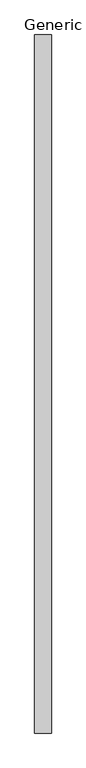
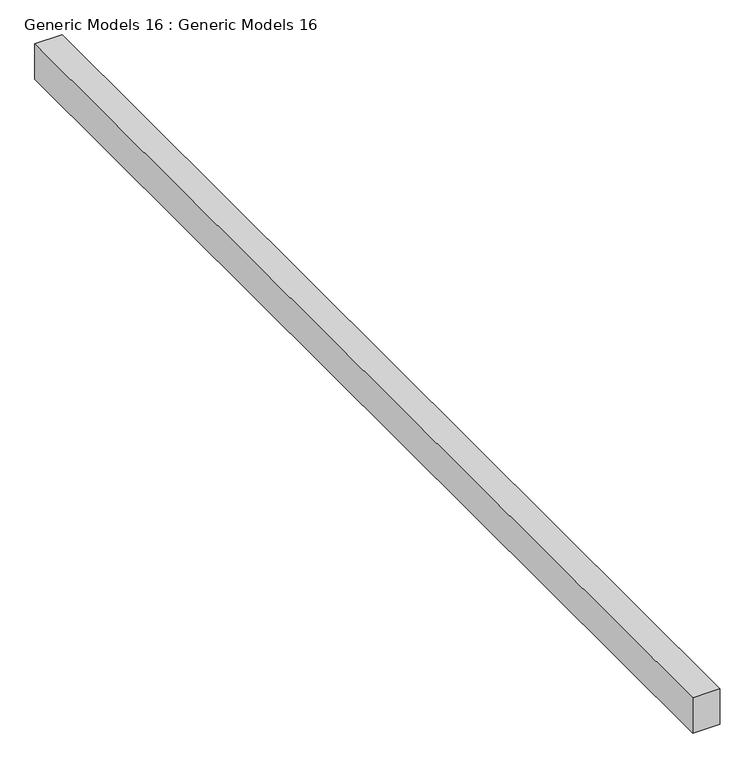
"""IFC4 building model written with IfcOpenShell, lengths in millimetres: proxy geometry, Generic Models 16 : Generic Models 16."""

from ifc_helpers import new_model, si_unit, frame, origin, place, context, project, spatial, polyline, outline, extrude, source, transform, mapped, element, save


def generic_models_16_generic_models_16_858d129d(model_context):
    return source(origin(), model_context, "Body", "SweptSolid", [
        extrude(outline(polyline([(-15581.438074, -5869.9774787), (-15581.438074, 6894.732482), (-15276.638074, 6894.732482), (-15276.638074, -5869.9774787), (-15581.438074, -5869.9774787)])), frame((0.0, 0.0, 26099.4794042), z_axis=(0.0, 0.0, 1.0), x_axis=(1.0, 0.0, 0.0)), (0.0, 0.0, 1.0), 418.1205958),
    ])


if __name__ == "__main__":
    model = new_model("IFC4")
    model_context = context("Model", 3, world=origin())
    ifc_project = project(units=[si_unit("LENGTHUNIT", "METRE", prefix="MILLI")], contexts=[model_context])
    site = spatial("IfcSite", under=ifc_project)
    building = spatial("IfcBuilding", under=site)
    placement = place(None, origin())
    generic_models_16_generic_models_16_shape = generic_models_16_generic_models_16_858d129d(model_context)
    element("IfcBuildingElementProxy", 1, Name="Generic Models 16 : Generic Models 16", ObjectType="Generic Models 16 : Generic Models 16", at=placement, inside=building, context=model_context, shape_type="MappedRepresentation", body=[
        mapped(generic_models_16_generic_models_16_shape, transform((0.0, 0.0, 0.0), x_axis=(1.0, 0.0, 0.0), y_axis=(0.0, 1.0, 0.0), z_axis=(0.0, 0.0, 1.0))),
    ])
    save(model, "model.ifc")
